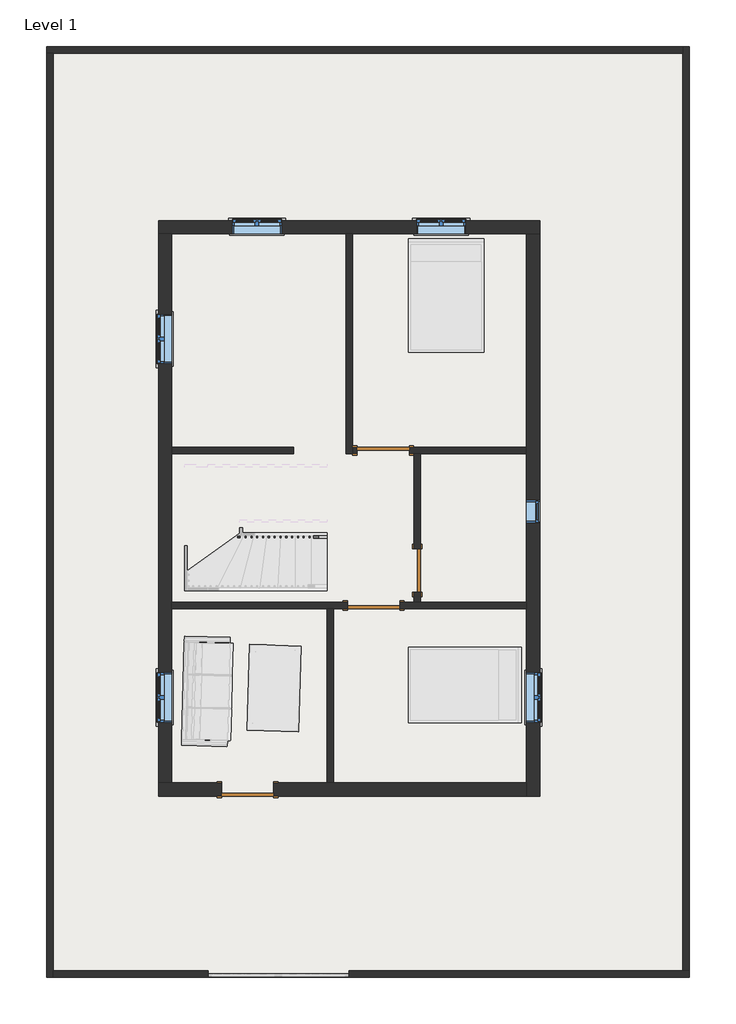
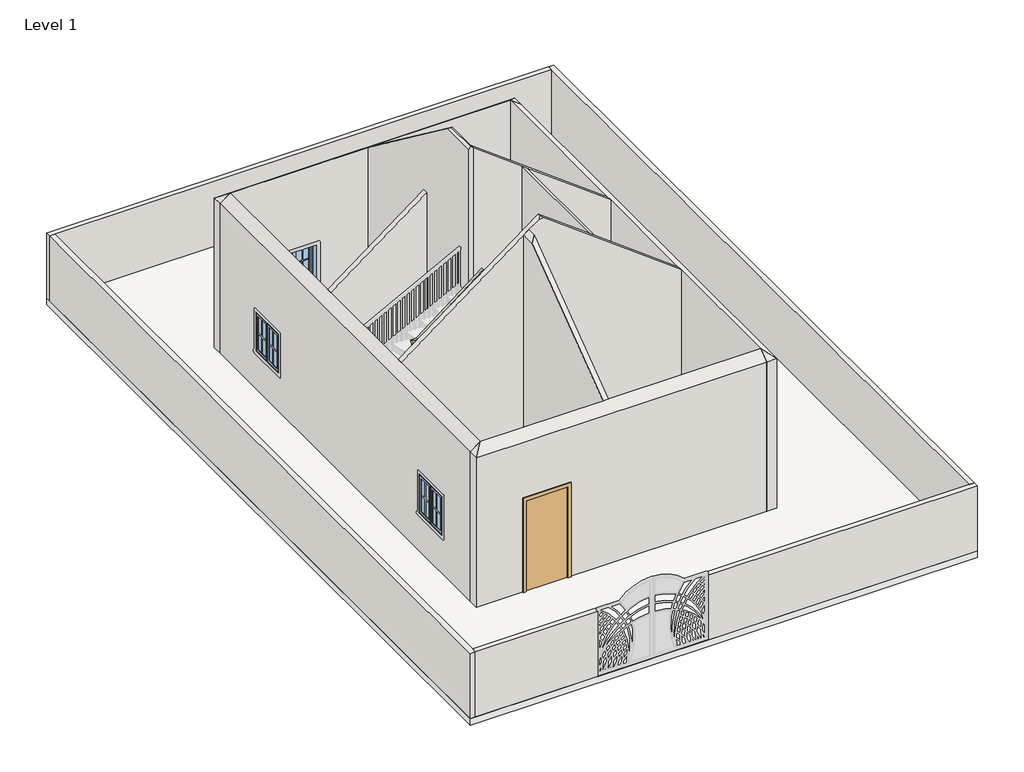
# One storey, part 1 of 2: 15 walls, 6 windows, 4 doors, 1 railing, 1 slab.
"""IFC4 building model written with IfcOpenShell, lengths in millimetres."""

from ifc_helpers import new_model, si_unit, frame, origin, origin_with_axes, place, context, project, spatial, polyline, outline, extrude, faceted_brep, transform, mapped, element, save
from components import door_d8f5dbb5, door_305aa2a5, door_e5f9f3c4, door_0ca8825f, window_aa618e30, window_339605e1

model = new_model("IFC4")

# Units and contexts
model_context = context("Model", 3, world=origin())
ifc_project = project(units=[si_unit("LENGTHUNIT", "METRE", prefix="MILLI")], contexts=[model_context])

# Site, building, storey
site = spatial("IfcSite", under=ifc_project)
building = spatial("IfcBuilding", under=site)
storey = spatial("IfcBuildingStorey", under=building, Name="Level 1", Elevation=0.0)

# Doors
placement = place(None, origin())
door_shape = door_d8f5dbb5(model_context)
element("IfcDoor", 1, ObjectType="Single-Flush : 30\" x 80\"", at=placement, inside=storey, context=model_context, shape_type="MappedRepresentation", body=[
    mapped(door_shape, transform((-82.2715692, -955.3070853, 0.0), x_axis=(0.0, -1.0, 0.0), y_axis=(1.0, 0.0, 0.0), z_axis=(0.0, 0.0, 1.0))),
])
door_2_shape = door_305aa2a5(model_context)
element("IfcDoor", 2, ObjectType="Single-Flush : 36\" x 84\"", at=placement, inside=storey, context=model_context, shape_type="MappedRepresentation", body=[
    mapped(door_2_shape, transform((-677.5332429, 1140.1929147, 0.0), x_axis=(-1.0, 0.0, 0.0), y_axis=(0.0, -1.0, 0.0), z_axis=(0.0, 0.0, 1.0))),
])
door_3_shape = door_e5f9f3c4(model_context)
element("IfcDoor", 3, ObjectType="Single-Flush : 36\" x 84\"", at=placement, inside=storey, context=model_context, shape_type="MappedRepresentation", body=[
    mapped(door_3_shape, transform((-842.6332429, -1564.9070853, 0.0), x_axis=(-1.0, 0.0, 0.0), y_axis=(0.0, -1.0, 0.0), z_axis=(0.0, 0.0, 1.0))),
])
door_4_shape = door_0ca8825f(model_context)
element("IfcDoor", 4, ObjectType="Single-Flush : 36\" x 84\"", at=placement, inside=storey, context=model_context, shape_type="MappedRepresentation", body=[
    mapped(door_4_shape, transform((-3047.6199167, -4784.3570853, 0.0), x_axis=(-1.0, 0.0, 0.0), y_axis=(0.0, -1.0, 0.0), z_axis=(0.0, 0.0, 1.0))),
])

# Railing
element("IfcRailing", 5, ObjectType="Handrail - Rectangular", at=placement, inside=storey, context=model_context, shape_type="SolidModel", body=[
    faceted_brep([(-1660.1449167, -396.5070853, 1083.7333333), (-1660.1449167, -396.5070853, 1019.4000346), (-1660.1449167, -345.7070853, 1019.4000346), (-1660.1449167, -345.7070853, 1083.7333333), (-3111.6766085, -396.5070853, 2211.6191036), (-3162.4766085, -396.5070853, 2186.7590024), (-3162.4766085, -345.7070853, 2186.7590024), (-3111.6766085, -345.7070853, 2211.6191036), (-3111.6766085, -396.5070853, 2414.6281882), (-3162.4766085, -396.5070853, 2363.8281882), (-3162.4766085, -345.7070853, 2363.8281882), (-3111.6766085, -345.7070853, 2414.6281882), (-3238.6766085, -396.5070853, 2414.6281882), (-3238.6766085, -396.5070853, 2363.8281882), (-3187.8766085, -345.7070853, 2363.8281882), (-3187.8766085, -345.7070853, 2414.6281882), (-3238.6766085, -269.5070853, 2414.6281882), (-3238.6766085, -240.3857515, 2363.8281882), (-3187.8766085, -240.3857515, 2363.8281882), (-3187.8766085, -269.5070853, 2414.6281882), (-3238.6766085, -142.5070853, 2631.5051451), (-3238.6766085, -91.7070853, 2617.7256424), (-3187.8766085, -91.7070853, 2617.7256424), (-3187.8766085, -142.5070853, 2631.5051451), (-3238.6766085, -142.5070853, 2834.5142297), (-3238.6766085, -91.7070853, 2783.7142297), (-3187.8766085, -91.7070853, 2783.7142297), (-3187.8766085, -142.5070853, 2834.5142297), (-3238.6766085, -15.5070853, 2834.5142297), (-3238.6766085, -15.5070853, 2783.7142297), (-3187.8766085, -66.3070853, 2783.7142297), (-3187.8766085, -66.3070853, 2834.5142297), (-3111.6766085, -15.5070853, 2834.5142297), (-3094.2599406, -15.5070853, 2783.7142297), (-3094.2599406, -66.3070853, 2783.7142297), (-3111.6766085, -66.3070853, 2834.5142297), (-1660.1449167, -15.5070853, 3962.4), (-1660.1449167, -66.3070853, 3962.4), (-1660.1449167, -66.3070853, 3898.0667013), (-1660.1449167, -15.5070853, 3898.0667013)], [[[0, 1, 2, 3]], [[1, 0, 4, 5]], [[2, 1, 5, 6]], [[3, 2, 6, 7]], [[0, 3, 7, 4]], [[5, 4, 8, 9]], [[6, 5, 9, 10]], [[7, 6, 10, 11]], [[4, 7, 11, 8]], [[9, 8, 12, 13]], [[10, 9, 13, 14]], [[11, 10, 14, 15]], [[8, 11, 15, 12]], [[13, 12, 16, 17]], [[14, 13, 17, 18]], [[15, 14, 18, 19]], [[12, 15, 19, 16]], [[17, 16, 20, 21]], [[18, 17, 21, 22]], [[19, 18, 22, 23]], [[16, 19, 23, 20]], [[21, 20, 24, 25]], [[22, 21, 25, 26]], [[23, 22, 26, 27]], [[20, 23, 27, 24]], [[25, 24, 28, 29]], [[26, 25, 29, 30]], [[27, 26, 30, 31]], [[24, 27, 31, 28]], [[29, 28, 32, 33]], [[30, 29, 33, 34]], [[31, 30, 34, 35]], [[28, 31, 35, 32]], [[36, 37, 38, 39]], [[33, 32, 36, 39]], [[34, 33, 39, 38]], [[35, 34, 38, 37]], [[32, 35, 37, 36]]]),
    extrude(outline(polyline([(3882.8316852, -1679.7516085), (3868.0292361, -1698.8016085), (2878.6666667, -1698.8016085), (2878.6666667, -1679.7516085), (3882.8316852, -1679.7516085)])), frame((0.0, -50.4320853, 0.0), z_axis=(0.0, 1.0, 0.0), x_axis=(0.0, 0.0, 1.0)), (0.0, 0.0, 1.0), 19.05),
    extrude(outline(polyline([(3803.8852902, -1781.3516085), (3789.0828411, -1800.4016085), (2878.6666667, -1800.4016085), (2878.6666667, -1781.3516085), (3803.8852902, -1781.3516085)])), frame((0.0, -50.4320853, 0.0), z_axis=(0.0, 1.0, 0.0), x_axis=(0.0, 0.0, 1.0)), (0.0, 0.0, 1.0), 19.05),
    extrude(outline(polyline([(3724.9388952, -1882.9516085), (3710.1364462, -1902.0016085), (2878.6666667, -1902.0016085), (2878.6666667, -1882.9516085), (3724.9388952, -1882.9516085)])), frame((0.0, -50.4320853, 0.0), z_axis=(0.0, 1.0, 0.0), x_axis=(0.0, 0.0, 1.0)), (0.0, 0.0, 1.0), 19.05),
    extrude(outline(polyline([(3645.9925003, -1984.5516085), (3631.1900512, -2003.6016085), (2709.3333333, -2003.6016085), (2709.3333333, -1984.5516085), (3645.9925003, -1984.5516085)])), frame((0.0, -50.4320853, 0.0), z_axis=(0.0, 1.0, 0.0), x_axis=(0.0, 0.0, 1.0)), (0.0, 0.0, 1.0), 19.05),
    extrude(outline(polyline([(3567.0461053, -2086.1516085), (3552.2436562, -2105.2016085), (2709.3333333, -2105.2016085), (2709.3333333, -2086.1516085), (3567.0461053, -2086.1516085)])), frame((0.0, -50.4320853, 0.0), z_axis=(0.0, 1.0, 0.0), x_axis=(0.0, 0.0, 1.0)), (0.0, 0.0, 1.0), 19.05),
    extrude(outline(polyline([(3488.0997103, -2187.7516085), (3473.2972613, -2206.8016085), (2709.3333333, -2206.8016085), (2709.3333333, -2187.7516085), (3488.0997103, -2187.7516085)])), frame((0.0, -50.4320853, 0.0), z_axis=(0.0, 1.0, 0.0), x_axis=(0.0, 0.0, 1.0)), (0.0, 0.0, 1.0), 19.05),
    extrude(outline(polyline([(3409.1533154, -2289.3516085), (3394.3508663, -2308.4016085), (2540.0, -2308.4016085), (2540.0, -2289.3516085), (3409.1533154, -2289.3516085)])), frame((0.0, -50.4320853, 0.0), z_axis=(0.0, 1.0, 0.0), x_axis=(0.0, 0.0, 1.0)), (0.0, 0.0, 1.0), 19.05),
    extrude(outline(polyline([(3330.2069204, -2390.9516085), (3315.4044713, -2410.0016085), (2540.0, -2410.0016085), (2540.0, -2390.9516085), (3330.2069204, -2390.9516085)])), frame((0.0, -50.4320853, 0.0), z_axis=(0.0, 1.0, 0.0), x_axis=(0.0, 0.0, 1.0)), (0.0, 0.0, 1.0), 19.05),
    extrude(outline(polyline([(3251.2605254, -2492.5516085), (3236.4580764, -2511.6016085), (2370.6666667, -2511.6016085), (2370.6666667, -2492.5516085), (3251.2605254, -2492.5516085)])), frame((0.0, -50.4320853, 0.0), z_axis=(0.0, 1.0, 0.0), x_axis=(0.0, 0.0, 1.0)), (0.0, 0.0, 1.0), 19.05),
    extrude(outline(polyline([(3172.3141304, -2594.1516085), (3157.5116814, -2613.2016085), (2370.6666667, -2613.2016085), (2370.6666667, -2594.1516085), (3172.3141304, -2594.1516085)])), frame((0.0, -50.4320853, 0.0), z_axis=(0.0, 1.0, 0.0), x_axis=(0.0, 0.0, 1.0)), (0.0, 0.0, 1.0), 19.05),
    extrude(outline(polyline([(3093.3677355, -2695.7516085), (3078.5652864, -2714.8016085), (2370.6666667, -2714.8016085), (2370.6666667, -2695.7516085), (3093.3677355, -2695.7516085)])), frame((0.0, -50.4320853, 0.0), z_axis=(0.0, 1.0, 0.0), x_axis=(0.0, 0.0, 1.0)), (0.0, 0.0, 1.0), 19.05),
    extrude(outline(polyline([(3014.4213405, -2797.3516085), (2999.6188914, -2816.4016085), (2201.3333333, -2816.4016085), (2201.3333333, -2797.3516085), (3014.4213405, -2797.3516085)])), frame((0.0, -50.4320853, 0.0), z_axis=(0.0, 1.0, 0.0), x_axis=(0.0, 0.0, 1.0)), (0.0, 0.0, 1.0), 19.05),
    extrude(outline(polyline([(2935.4749455, -2898.9516085), (2920.6724965, -2918.0016085), (2201.3333333, -2918.0016085), (2201.3333333, -2898.9516085), (2935.4749455, -2898.9516085)])), frame((0.0, -50.4320853, 0.0), z_axis=(0.0, 1.0, 0.0), x_axis=(0.0, 0.0, 1.0)), (0.0, 0.0, 1.0), 19.05),
    extrude(outline(polyline([(2856.5285506, -3000.5516085), (2841.7261015, -3019.6016085), (2032.0, -3019.6016085), (2032.0, -3000.5516085), (2856.5285506, -3000.5516085)])), frame((0.0, -50.4320853, 0.0), z_axis=(0.0, 1.0, 0.0), x_axis=(0.0, 0.0, 1.0)), (0.0, 0.0, 1.0), 19.05),
    extrude(outline(polyline([(2777.5821556, -3102.1516085), (2762.7797065, -3121.2016085), (2032.0, -3121.2016085), (2032.0, -3102.1516085), (2777.5821556, -3102.1516085)])), frame((0.0, -50.4320853, 0.0), z_axis=(0.0, 1.0, 0.0), x_axis=(0.0, 0.0, 1.0)), (0.0, 0.0, 1.0), 19.05),
    extrude(outline(polyline([(-3203.7516085, -75.8320853), (-3222.8016085, -75.8320853), (-3222.8016085, -56.7820853), (-3203.7516085, -56.7820853), (-3203.7516085, -75.8320853)])), frame((0.0, 0.0, 1693.3333333), z_axis=(0.0, 0.0, 1.0), x_axis=(1.0, 0.0, 0.0)), (0.0, 0.0, 1.0), 1090.3808964),
    extrude(outline(polyline([(-177.4320853, 2471.3336964), (-158.3820853, 2503.86524), (-158.3820853, 1524.0), (-177.4320853, 1524.0), (-177.4320853, 2471.3336964)])), frame((-3222.8016085, 0.0, 0.0), z_axis=(1.0, 0.0, 0.0), x_axis=(0.0, 1.0, 0.0)), (0.0, 0.0, 1.0), 19.05),
    extrude(outline(polyline([(-279.0320853, 2297.8321309), (-259.9820853, 2330.3636744), (-259.9820853, 1354.6666667), (-279.0320853, 1354.6666667), (-279.0320853, 2297.8321309)])), frame((-3222.8016085, 0.0, 0.0), z_axis=(1.0, 0.0, 0.0), x_axis=(0.0, 1.0, 0.0)), (0.0, 0.0, 1.0), 19.05),
    extrude(outline(polyline([(-3174.6199167, -361.5820853), (-3174.6199167, -380.6320853), (-3193.6699167, -380.6320853), (-3193.6699167, -361.5820853), (-3174.6199167, -361.5820853)])), frame((0.0, 0.0, 1185.3333333), z_axis=(0.0, 0.0, 1.0), x_axis=(1.0, 0.0, 0.0)), (0.0, 0.0, 1.0), 1178.4948549),
    extrude(outline(polyline([(2117.2483397, -3073.0199167), (2132.0507888, -3092.0699167), (1016.0, -3092.0699167), (1016.0, -3073.0199167), (2117.2483397, -3073.0199167)])), frame((0.0, -380.6320853, 0.0), z_axis=(0.0, 1.0, 0.0), x_axis=(0.0, 0.0, 1.0)), (0.0, 0.0, 1.0), 19.05),
    extrude(outline(polyline([(2038.3019447, -2971.4199167), (2053.1043938, -2990.4699167), (1016.0, -2990.4699167), (1016.0, -2971.4199167), (2038.3019447, -2971.4199167)])), frame((0.0, -380.6320853, 0.0), z_axis=(0.0, 1.0, 0.0), x_axis=(0.0, 0.0, 1.0)), (0.0, 0.0, 1.0), 19.05),
    extrude(outline(polyline([(1959.3555498, -2869.8199167), (1974.1579988, -2888.8699167), (846.6666667, -2888.8699167), (846.6666667, -2869.8199167), (1959.3555498, -2869.8199167)])), frame((0.0, -380.6320853, 0.0), z_axis=(0.0, 1.0, 0.0), x_axis=(0.0, 0.0, 1.0)), (0.0, 0.0, 1.0), 19.05),
    extrude(outline(polyline([(1880.4091548, -2768.2199167), (1895.2116039, -2787.2699167), (846.6666667, -2787.2699167), (846.6666667, -2768.2199167), (1880.4091548, -2768.2199167)])), frame((0.0, -380.6320853, 0.0), z_axis=(0.0, 1.0, 0.0), x_axis=(0.0, 0.0, 1.0)), (0.0, 0.0, 1.0), 19.05),
    extrude(outline(polyline([(1801.4627598, -2666.6199167), (1816.2652089, -2685.6699167), (677.3333333, -2685.6699167), (677.3333333, -2666.6199167), (1801.4627598, -2666.6199167)])), frame((0.0, -380.6320853, 0.0), z_axis=(0.0, 1.0, 0.0), x_axis=(0.0, 0.0, 1.0)), (0.0, 0.0, 1.0), 19.05),
    extrude(outline(polyline([(1722.5163649, -2565.0199167), (1737.3188139, -2584.0699167), (677.3333333, -2584.0699167), (677.3333333, -2565.0199167), (1722.5163649, -2565.0199167)])), frame((0.0, -380.6320853, 0.0), z_axis=(0.0, 1.0, 0.0), x_axis=(0.0, 0.0, 1.0)), (0.0, 0.0, 1.0), 19.05),
    extrude(outline(polyline([(1643.5699699, -2463.4199167), (1658.3724189, -2482.4699167), (508.0, -2482.4699167), (508.0, -2463.4199167), (1643.5699699, -2463.4199167)])), frame((0.0, -380.6320853, 0.0), z_axis=(0.0, 1.0, 0.0), x_axis=(0.0, 0.0, 1.0)), (0.0, 0.0, 1.0), 19.05),
    extrude(outline(polyline([(1564.6235749, -2361.8199167), (1579.426024, -2380.8699167), (508.0, -2380.8699167), (508.0, -2361.8199167), (1564.6235749, -2361.8199167)])), frame((0.0, -380.6320853, 0.0), z_axis=(0.0, 1.0, 0.0), x_axis=(0.0, 0.0, 1.0)), (0.0, 0.0, 1.0), 19.05),
    extrude(outline(polyline([(1485.6771799, -2260.2199167), (1500.479629, -2279.2699167), (508.0, -2279.2699167), (508.0, -2260.2199167), (1485.6771799, -2260.2199167)])), frame((0.0, -380.6320853, 0.0), z_axis=(0.0, 1.0, 0.0), x_axis=(0.0, 0.0, 1.0)), (0.0, 0.0, 1.0), 19.05),
    extrude(outline(polyline([(1406.730785, -2158.6199167), (1421.533234, -2177.6699167), (338.6666667, -2177.6699167), (338.6666667, -2158.6199167), (1406.730785, -2158.6199167)])), frame((0.0, -380.6320853, 0.0), z_axis=(0.0, 1.0, 0.0), x_axis=(0.0, 0.0, 1.0)), (0.0, 0.0, 1.0), 19.05),
    extrude(outline(polyline([(1327.78439, -2057.0199167), (1342.5868391, -2076.0699167), (338.6666667, -2076.0699167), (338.6666667, -2057.0199167), (1327.78439, -2057.0199167)])), frame((0.0, -380.6320853, 0.0), z_axis=(0.0, 1.0, 0.0), x_axis=(0.0, 0.0, 1.0)), (0.0, 0.0, 1.0), 19.05),
    extrude(outline(polyline([(1248.837995, -1955.4199167), (1263.6404441, -1974.4699167), (338.6666667, -1974.4699167), (338.6666667, -1955.4199167), (1248.837995, -1955.4199167)])), frame((0.0, -380.6320853, 0.0), z_axis=(0.0, 1.0, 0.0), x_axis=(0.0, 0.0, 1.0)), (0.0, 0.0, 1.0), 19.05),
    extrude(outline(polyline([(1169.8916001, -1853.8199167), (1184.6940491, -1872.8699167), (169.3333333, -1872.8699167), (169.3333333, -1853.8199167), (1169.8916001, -1853.8199167)])), frame((0.0, -380.6320853, 0.0), z_axis=(0.0, 1.0, 0.0), x_axis=(0.0, 0.0, 1.0)), (0.0, 0.0, 1.0), 19.05),
    extrude(outline(polyline([(1090.9452051, -1752.2199167), (1105.7476541, -1771.2699167), (169.3333333, -1771.2699167), (169.3333333, -1752.2199167), (1090.9452051, -1752.2199167)])), frame((0.0, -380.6320853, 0.0), z_axis=(0.0, 1.0, 0.0), x_axis=(0.0, 0.0, 1.0)), (0.0, 0.0, 1.0), 19.05),
    extrude(outline(polyline([(-3203.7516085, -50.4320853), (-3222.8016085, -50.4320853), (-3222.8016085, -31.3820853), (-3203.7516085, -31.3820853), (-3203.7516085, -50.4320853)])), frame((0.0, 0.0, 1862.6666667), z_axis=(0.0, 0.0, 1.0), x_axis=(1.0, 0.0, 0.0)), (0.0, 0.0, 1.0), 921.0475631),
    extrude(outline(polyline([(-3203.7516085, -361.5820853), (-3203.7516085, -380.6320853), (-3222.8016085, -380.6320853), (-3222.8016085, -361.5820853), (-3203.7516085, -361.5820853)])), frame((0.0, 0.0, 1185.3333333), z_axis=(0.0, 0.0, 1.0), x_axis=(1.0, 0.0, 0.0)), (0.0, 0.0, 1.0), 1178.4948549),
    extrude(outline(polyline([(3898.0667013, -1660.1449167), (3883.2642523, -1679.1949167), (2878.6666667, -1679.1949167), (2878.6666667, -1660.1449167), (3898.0667013, -1660.1449167)])), frame((0.0, -50.4320853, 0.0), z_axis=(0.0, 1.0, 0.0), x_axis=(0.0, 0.0, 1.0)), (0.0, 0.0, 1.0), 19.05),
    extrude(outline(polyline([(1019.4000346, -1660.1449167), (1034.2024837, -1679.1949167), (169.3333333, -1679.1949167), (169.3333333, -1660.1449167), (1019.4000346, -1660.1449167)])), frame((0.0, -380.6320853, 0.0), z_axis=(0.0, 1.0, 0.0), x_axis=(0.0, 0.0, 1.0)), (0.0, 0.0, 1.0), 19.05),
])

# Slab
element("IfcSlab", 6, ObjectType="Generic - 12\"", at=placement, inside=storey, context=model_context, shape_type="SweptSolid", body=[
    extrude(outline(polyline([(4675.3638952, 8200.4974943), (4675.3638952, -8068.2025057), (-6564.1361048, -8068.2025057), (-6564.1361048, 8200.4974943), (4675.3638952, 8200.4974943)])), frame((0.0, 0.0, -152.4), z_axis=(0.0, 0.0, 1.0), x_axis=(1.0, 0.0, 0.0)), (0.0, 0.0, 1.0), 152.4),
])

# Walls
element("IfcWall", 7, ObjectType="WALL4.5\"", at=placement, inside=storey, context=model_context, shape_type="Brep", body=[
    faceted_brep([(-1329.9449167, 4931.1429147, 0.0), (-1329.9449167, 1083.0429147, 0.0), (-1329.9449167, 1083.0429147, 5962.65), (-1329.9449167, 1883.1429147, 5962.65), (-1329.9449167, 4931.1429147, 3676.65), (-1215.6449167, 4931.1429147, 0.0), (-1215.6449167, 4931.1429147, 3676.65), (-1215.6449167, 1883.1429147, 5962.65), (-1215.6449167, 1197.3429147, 5962.65), (-1215.6449167, 1083.0429147, 5962.65), (-1215.6449167, 1083.0429147, 0.0), (-1215.6449167, 1197.3429147, 0.0), (-1272.7949167, 1083.0429147, 6005.5125), (-1272.7949167, 1825.9929147, 6005.5125)], [[[0, 1, 2, 3, 4]], [[5, 6, 7, 8, 9, 10, 11]], [[1, 0, 5, 11, 10]], [[0, 4, 6, 5]], [[2, 1, 10, 9, 12]], [[4, 3, 13, 7, 6]], [[3, 2, 12, 13]], [[12, 9, 8, 7, 13]]]),
])
element("IfcWall", 8, ObjectType="WALL4.5\"", at=placement, inside=storey, context=model_context, shape_type="Brep", body=[
    faceted_brep([(-1215.6449167, 1083.0429147, 0.0), (-1134.7332429, 1083.0429147, 0.0), (-1134.7332429, 1083.0429147, 2133.6), (-220.3332429, 1083.0429147, 2133.6), (-220.3332429, 1083.0429147, 0.0), (-139.4215692, 1083.0429147, 0.0), (-25.1215692, 1083.0429147, 0.0), (1832.3550833, 1083.0429147, 0.0), (1832.3550833, 1083.0429147, 3676.65), (-25.1215692, 1083.0429147, 5069.7574894), (-139.4215692, 1083.0429147, 5155.4824894), (-1215.6449167, 1083.0429147, 5962.65), (-1134.7332429, 1197.3429147, 2133.6), (-1134.7332429, 1197.3429147, 0.0), (-1215.6449167, 1197.3429147, 0.0), (-1215.6449167, 1197.3429147, 5962.65), (1832.3550833, 1197.3429147, 3676.65), (1832.3550833, 1197.3429147, 0.0), (-220.3332429, 1197.3429147, 0.0), (-220.3332429, 1197.3429147, 2133.6)], [[[0, 1, 2, 3, 4, 5, 6, 7, 8, 9, 10, 11]], [[12, 13, 14, 15, 16, 17, 18, 19]], [[18, 17, 7, 6, 5, 4]], [[14, 13, 1, 0]], [[0, 11, 15, 14]], [[8, 7, 17, 16]], [[2, 1, 13, 12]], [[3, 2, 12, 19]], [[4, 3, 19, 18]], [[11, 10, 9, 8, 16, 15]]]),
])
element("IfcWall", 9, ObjectType="WALL4.5\"", at=placement, inside=storey, context=model_context, shape_type="SweptSolid", body=[
    extrude(outline(polyline([(0.0, -4377.9449167), (0.0, -2244.3449167), (5276.85, -2244.3449167), (3676.65, -4377.9449167), (0.0, -4377.9449167)])), frame((0.0, 1083.0429147, 0.0), z_axis=(0.0, 1.0, 0.0), x_axis=(0.0, 0.0, 1.0)), (0.0, 0.0, 1.0), 114.3),
])
element("IfcWall", 10, ObjectType="WALL4.5\"", at=placement, inside=storey, context=model_context, shape_type="Brep", body=[
    faceted_brep([(-139.4215692, -1336.3070853, 2032.0), (-139.4215692, -1336.3070853, 0.0), (-139.4215692, -1507.7570853, 0.0), (-139.4215692, -1507.7570853, 5155.4824894), (-139.4215692, 1083.0429147, 5155.4824894), (-139.4215692, 1083.0429147, 0.0), (-139.4215692, -574.3070853, 0.0), (-139.4215692, -574.3070853, 2032.0), (-25.1215692, -1507.7570853, 0.0), (-25.1215692, -1336.3070853, 0.0), (-25.1215692, -1336.3070853, 2032.0), (-25.1215692, -574.3070853, 2032.0), (-25.1215692, -574.3070853, 0.0), (-25.1215692, 1083.0429147, 0.0), (-25.1215692, 1083.0429147, 5069.7574894), (-25.1215692, -1507.7570853, 5069.7574894)], [[[0, 1, 2, 3, 4, 5, 6, 7]], [[8, 9, 10, 11, 12, 13, 14, 15]], [[6, 5, 13, 12]], [[2, 1, 9, 8]], [[5, 4, 14, 13]], [[3, 2, 8, 15]], [[10, 9, 1, 0]], [[11, 10, 0, 7]], [[12, 11, 7, 6]], [[4, 3, 15, 14]]]),
])
element("IfcWall", 11, ObjectType="WALL4.5\"", at=placement, inside=storey, context=model_context, shape_type="Brep", body=[
    faceted_brep([(-4377.9449167, -1622.0570853, 0.0), (-1660.1449167, -1622.0570853, 0.0), (-1545.8449167, -1622.0570853, 0.0), (-1299.8332429, -1622.0570853, 0.0), (-1299.8332429, -1622.0570853, 2133.6), (-385.4332429, -1622.0570853, 2133.6), (-385.4332429, -1622.0570853, 0.0), (1832.3550833, -1622.0570853, 0.0), (1832.3550833, -1622.0570853, 3676.65), (-1215.6449167, -1622.0570853, 5962.65), (-1329.9449167, -1622.0570853, 5962.65), (-1545.8449167, -1622.0570853, 5800.725), (-1660.1449167, -1622.0570853, 5715.0), (-4377.9449167, -1622.0570853, 3676.65), (-1299.8332429, -1507.7570853, 2133.6), (-1299.8332429, -1507.7570853, 0.0), (-4377.9449167, -1507.7570853, 0.0), (-4377.9449167, -1507.7570853, 3676.65), (-1272.7949167, -1507.7570853, 6005.5125), (-139.4215692, -1507.7570853, 5155.4824894), (-25.1215692, -1507.7570853, 5069.7574894), (1832.3550833, -1507.7570853, 3676.65), (1832.3550833, -1507.7570853, 0.0), (-25.1215692, -1507.7570853, 0.0), (-139.4215692, -1507.7570853, 0.0), (-385.4332429, -1507.7570853, 0.0), (-385.4332429, -1507.7570853, 2133.6), (-1272.7949167, -1564.9070853, 6005.5125)], [[[0, 1, 2, 3, 4, 5, 6, 7, 8, 9, 10, 11, 12, 13]], [[14, 15, 16, 17, 18, 19, 20, 21, 22, 23, 24, 25, 26]], [[16, 15, 3, 2, 1, 0]], [[25, 24, 23, 22, 7, 6]], [[8, 7, 22, 21]], [[0, 13, 17, 16]], [[4, 3, 15, 14]], [[5, 4, 14, 26]], [[6, 5, 26, 25]], [[13, 12, 11, 10, 27, 18, 17]], [[10, 9, 27]], [[9, 8, 21, 20, 19, 18, 27]]]),
])
element("IfcWall", 12, ObjectType="WALL4.5\"", at=placement, inside=storey, context=model_context, shape_type="Brep", body=[
    faceted_brep([(-1660.1449167, -1622.0570853, 0.0), (-1660.1449167, -4670.0570853, 0.0), (-1660.1449167, -4670.0570853, 3676.65), (-1660.1449167, -1952.2570853, 5715.0), (-1660.1449167, -1622.0570853, 5715.0), (-1545.8449167, -1622.0570853, 0.0), (-1545.8449167, -1622.0570853, 5800.725), (-1545.8449167, -1837.9570853, 5800.725), (-1545.8449167, -4670.0570853, 3676.65), (-1545.8449167, -4670.0570853, 0.0)], [[[0, 1, 2, 3, 4]], [[5, 6, 7, 8, 9]], [[1, 0, 5, 9]], [[2, 1, 9, 8]], [[0, 4, 6, 5]], [[4, 3, 7, 6]], [[3, 2, 8, 7]]]),
])
element("IfcWall", 13, ObjectType="WALL4.5\"", at=placement, inside=storey, context=model_context, shape_type="Brep", body=[
    faceted_brep([(-6564.1361048, 8086.1974943, 0.0), (-6449.8361048, 8086.1974943, 0.0), (4561.0638952, 8086.1974943, 0.0), (4561.0638952, 8086.1974943, 1524.0), (-6449.8361048, 8086.1974943, 1524.0), (-6564.1361048, 8086.1974943, 1524.0), (-6564.1361048, 8200.4974943, 0.0), (-6564.1361048, 8200.4974943, 1524.0), (4561.0638952, 8200.4974943, 1524.0), (4561.0638952, 8200.4974943, 0.0)], [[[0, 1, 2, 3, 4, 5]], [[6, 7, 8, 9]], [[2, 1, 0, 6, 9]], [[5, 4, 3, 8, 7]], [[0, 5, 7, 6]], [[3, 2, 9, 8]]]),
])
element("IfcWall", 14, ObjectType="WALL4.5\"", at=placement, inside=storey, context=model_context, shape_type="Brep", body=[
    faceted_brep([(-6449.8361048, -8068.2025057, 0.0), (-6449.8361048, -7953.9025057, 0.0), (-6449.8361048, 8086.1974943, 0.0), (-6449.8361048, 8086.1974943, 1524.0), (-6449.8361048, -7953.9025057, 1524.0), (-6449.8361048, -8068.2025057, 1524.0), (-6564.1361048, -8068.2025057, 0.0), (-6564.1361048, -8068.2025057, 1524.0), (-6564.1361048, 8086.1974943, 1524.0), (-6564.1361048, 8086.1974943, 0.0)], [[[0, 1, 2, 3, 4, 5]], [[6, 7, 8, 9]], [[2, 1, 0, 6, 9]], [[5, 4, 3, 8, 7]], [[0, 5, 7, 6]], [[3, 2, 9, 8]]]),
])
element("IfcWall", 15, ObjectType="WALL4.5\"", at=placement, inside=storey, context=model_context, shape_type="Brep", body=[
    faceted_brep([(4675.3638952, -7953.9025057, 0.0), (4561.0638952, -7953.9025057, 0.0), (-1274.5861048, -7953.9025057, 0.0), (-1274.5861048, -7953.9025057, 1524.0), (4561.0638952, -7953.9025057, 1524.0), (4675.3638952, -7953.9025057, 1524.0), (4675.3638952, -8068.2025057, 0.0), (4675.3638952, -8068.2025057, 1524.0), (-1274.5861048, -8068.2025057, 1524.0), (-1274.5861048, -8068.2025057, 0.0)], [[[0, 1, 2, 3, 4, 5]], [[6, 7, 8, 9]], [[2, 1, 0, 6, 9]], [[3, 2, 9, 8]], [[5, 4, 3, 8, 7]], [[0, 5, 7, 6]]]),
])
element("IfcWall", 16, ObjectType="WALL4.5\"", at=placement, inside=storey, context=model_context, shape_type="Brep", body=[
    faceted_brep([(4561.0638952, 8200.4974943, 0.0), (4561.0638952, 8086.1974943, 0.0), (4561.0638952, -7953.9025057, 0.0), (4561.0638952, -7953.9025057, 1524.0), (4561.0638952, 8086.1974943, 1524.0), (4561.0638952, 8200.4974943, 1524.0), (4675.3638952, 8200.4974943, 0.0), (4675.3638952, 8200.4974943, 1524.0), (4675.3638952, -7953.9025057, 1524.0), (4675.3638952, -7953.9025057, 0.0)], [[[0, 1, 2, 3, 4, 5]], [[6, 7, 8, 9]], [[2, 1, 0, 6, 9]], [[5, 4, 3, 8, 7]], [[0, 5, 7, 6]], [[3, 2, 9, 8]]]),
])
element("IfcWall", 17, ObjectType="WALL4.5\"", at=placement, inside=storey, context=model_context, shape_type="SweptSolid", body=[
    extrude(outline(polyline([(-6449.8361048, -7953.9025057), (-3739.7699167, -7953.9025057), (-3739.7699167, -8068.2025057), (-6449.8361048, -8068.2025057), (-6449.8361048, -7953.9025057)])), origin_with_axes(), (0.0, 0.0, 1.0), 1524.0),
])
element("IfcWall", 18, ObjectType="WALL9\"", at=placement, inside=storey, context=model_context, shape_type="Brep", body=[
    faceted_brep([(-4606.5449167, 4931.1429147, 0.0), (-4377.9449167, 4931.1429147, 0.0), (-1329.9449167, 4931.1429147, 0.0), (-1215.6449167, 4931.1429147, 0.0), (1832.3550833, 4931.1429147, 0.0), (2060.9550833, 4931.1429147, 0.0), (2060.9550833, 4931.1429147, 3505.2), (1832.3550833, 4931.1429147, 3676.65), (-1215.6449167, 4931.1429147, 3676.65), (-1329.9449167, 4931.1429147, 3676.65), (-4377.9449167, 4931.1429147, 3676.65), (-4606.5449167, 4931.1429147, 3505.2), (-2450.7199167, 4931.1429147, 1828.8), (-2450.7199167, 4931.1429147, 914.4), (-3314.3199167, 4931.1429147, 914.4), (-3314.3199167, 4931.1429147, 1828.8), (768.7300833, 4931.1429147, 1828.8), (768.7300833, 4931.1429147, 914.4), (-94.8699167, 4931.1429147, 914.4), (-94.8699167, 4931.1429147, 1828.8), (-4606.5449167, 5159.7429147, 0.0), (-4606.5449167, 5159.7429147, 3505.2), (2060.9550833, 5159.7429147, 3505.2), (2060.9550833, 5159.7429147, 0.0), (-2450.7199167, 5159.7429147, 1828.8), (-3314.3199167, 5159.7429147, 1828.8), (-3314.3199167, 5159.7429147, 914.4), (-2450.7199167, 5159.7429147, 914.4), (768.7300833, 5159.7429147, 1828.8), (-94.8699167, 5159.7429147, 1828.8), (-94.8699167, 5159.7429147, 914.4), (768.7300833, 5159.7429147, 914.4)], [[[0, 1, 2, 3, 4, 5, 6, 7, 8, 9, 10, 11], [12, 13, 14, 15], [16, 17, 18, 19]], [[20, 21, 22, 23], [24, 25, 26, 27], [28, 29, 30, 31]], [[5, 4, 3, 2, 1, 0, 20, 23]], [[6, 5, 23, 22]], [[0, 11, 21, 20]], [[13, 12, 24, 27]], [[14, 13, 27, 26]], [[15, 14, 26, 25]], [[12, 15, 25, 24]], [[17, 16, 28, 31]], [[18, 17, 31, 30]], [[19, 18, 30, 29]], [[16, 19, 29, 28]], [[11, 10, 21]], [[10, 9, 8, 7, 22, 21]], [[7, 6, 22]]]),
])
element("IfcWall", 19, ObjectType="WALL9\"", at=placement, inside=storey, context=model_context, shape_type="Brep", body=[
    faceted_brep([(1832.3550833, 4931.1429147, 0.0), (1832.3550833, 1197.3429147, 0.0), (1832.3550833, 1083.0429147, 0.0), (1832.3550833, -1507.7570853, 0.0), (1832.3550833, -1622.0570853, 0.0), (1832.3550833, -4670.0570853, 0.0), (1832.3550833, -4898.6570853, 0.0), (1832.3550833, -4898.6570853, 3505.2), (1832.3550833, -4670.0570853, 3676.65), (1832.3550833, -1622.0570853, 3676.65), (1832.3550833, -1507.7570853, 3676.65), (1832.3550833, 1083.0429147, 3676.65), (1832.3550833, 1197.3429147, 3676.65), (1832.3550833, 4931.1429147, 3676.65), (1832.3550833, -129.8070853, 1524.0), (1832.3550833, -129.8070853, 914.4), (1832.3550833, 276.5929147, 914.4), (1832.3550833, 276.5929147, 1524.0), (1832.3550833, -3606.4320853, 1828.8), (1832.3550833, -3606.4320853, 914.4), (1832.3550833, -2742.8320853, 914.4), (1832.3550833, -2742.8320853, 1828.8), (2060.9550833, 4931.1429147, 0.0), (2060.9550833, 4931.1429147, 3505.2), (2060.9550833, -4898.6570853, 3505.2), (2060.9550833, -4898.6570853, 0.0), (2060.9550833, -129.8070853, 1524.0), (2060.9550833, 276.5929147, 1524.0), (2060.9550833, 276.5929147, 914.4), (2060.9550833, -129.8070853, 914.4), (2060.9550833, -3606.4320853, 1828.8), (2060.9550833, -2742.8320853, 1828.8), (2060.9550833, -2742.8320853, 914.4), (2060.9550833, -3606.4320853, 914.4)], [[[0, 1, 2, 3, 4, 5, 6, 7, 8, 9, 10, 11, 12, 13], [14, 15, 16, 17], [18, 19, 20, 21]], [[22, 23, 24, 25], [26, 27, 28, 29], [30, 31, 32, 33]], [[6, 5, 4, 3, 2, 1, 0, 22, 25]], [[0, 13, 23, 22]], [[7, 6, 25, 24]], [[15, 14, 26, 29]], [[16, 15, 29, 28]], [[17, 16, 28, 27]], [[14, 17, 27, 26]], [[19, 18, 30, 33]], [[20, 19, 33, 32]], [[21, 20, 32, 31]], [[18, 21, 31, 30]], [[13, 12, 11, 10, 9, 8, 24, 23]], [[8, 7, 24]]]),
])
element("IfcWall", 20, ObjectType="WALL9\"", at=placement, inside=storey, context=model_context, shape_type="Brep", body=[
    faceted_brep([(-3504.8199167, -4670.0570853, 2133.6), (-3504.8199167, -4670.0570853, 0.0), (-4377.9449167, -4670.0570853, 0.0), (-4606.5449167, -4670.0570853, 0.0), (-4606.5449167, -4670.0570853, 3505.2), (-4377.9449167, -4670.0570853, 3676.65), (-1660.1449167, -4670.0570853, 3676.65), (-1545.8449167, -4670.0570853, 3676.65), (1832.3550833, -4670.0570853, 3676.65), (1832.3550833, -4670.0570853, 0.0), (-1545.8449167, -4670.0570853, 0.0), (-1660.1449167, -4670.0570853, 0.0), (-2590.4199167, -4670.0570853, 0.0), (-2590.4199167, -4670.0570853, 2133.6), (-4606.5449167, -4898.6570853, 0.0), (-3504.8199167, -4898.6570853, 0.0), (-3504.8199167, -4898.6570853, 2133.6), (-2590.4199167, -4898.6570853, 2133.6), (-2590.4199167, -4898.6570853, 0.0), (1832.3550833, -4898.6570853, 0.0), (1832.3550833, -4898.6570853, 3505.2), (-4606.5449167, -4898.6570853, 3505.2)], [[[0, 1, 2, 3, 4, 5, 6, 7, 8, 9, 10, 11, 12, 13]], [[14, 15, 16, 17, 18, 19, 20, 21]], [[3, 2, 1, 15, 14]], [[12, 11, 10, 9, 19, 18]], [[9, 8, 20, 19]], [[4, 3, 14, 21]], [[16, 15, 1, 0]], [[17, 16, 0, 13]], [[18, 17, 13, 12]], [[8, 7, 6, 5, 21, 20]], [[5, 4, 21]]]),
])
element("IfcWall", 21, ObjectType="WALL9\"", at=placement, inside=storey, context=model_context, shape_type="Brep", body=[
    faceted_brep([(-4377.9449167, -4670.0570853, 0.0), (-4377.9449167, -1622.0570853, 0.0), (-4377.9449167, -1507.7570853, 0.0), (-4377.9449167, 1083.0429147, 0.0), (-4377.9449167, 1197.3429147, 0.0), (-4377.9449167, 4931.1429147, 0.0), (-4377.9449167, 4931.1429147, 3676.65), (-4377.9449167, 1197.3429147, 3676.65), (-4377.9449167, 1083.0429147, 3676.65), (-4377.9449167, -1507.7570853, 3676.65), (-4377.9449167, -1622.0570853, 3676.65), (-4377.9449167, -4670.0570853, 3676.65), (-4377.9449167, 3524.6179147, 1828.8), (-4377.9449167, 3524.6179147, 914.4), (-4377.9449167, 2661.0179147, 914.4), (-4377.9449167, 2661.0179147, 1828.8), (-4377.9449167, -2742.8320853, 1828.8), (-4377.9449167, -2742.8320853, 914.4), (-4377.9449167, -3606.4320853, 914.4), (-4377.9449167, -3606.4320853, 1828.8), (-4606.5449167, -4670.0570853, 0.0), (-4606.5449167, -4670.0570853, 3505.2), (-4606.5449167, 4931.1429147, 3505.2), (-4606.5449167, 4931.1429147, 0.0), (-4606.5449167, 3524.6179147, 1828.8), (-4606.5449167, 2661.0179147, 1828.8), (-4606.5449167, 2661.0179147, 914.4), (-4606.5449167, 3524.6179147, 914.4), (-4606.5449167, -2742.8320853, 1828.8), (-4606.5449167, -3606.4320853, 1828.8), (-4606.5449167, -3606.4320853, 914.4), (-4606.5449167, -2742.8320853, 914.4)], [[[0, 1, 2, 3, 4, 5, 6, 7, 8, 9, 10, 11], [12, 13, 14, 15], [16, 17, 18, 19]], [[20, 21, 22, 23], [24, 25, 26, 27], [28, 29, 30, 31]], [[5, 4, 3, 2, 1, 0, 20, 23]], [[0, 11, 21, 20]], [[6, 5, 23, 22]], [[13, 12, 24, 27]], [[14, 13, 27, 26]], [[15, 14, 26, 25]], [[12, 15, 25, 24]], [[17, 16, 28, 31]], [[18, 17, 31, 30]], [[19, 18, 30, 29]], [[16, 19, 29, 28]], [[11, 10, 9, 8, 7, 6, 22, 21]]]),
])

# Windows
window_shape = window_aa618e30(model_context)
element("IfcWindow", 22, ObjectType="Fixed : 16\" x 24\"", at=placement, inside=storey, context=model_context, shape_type="MappedRepresentation", body=[
    mapped(window_shape, transform((1946.6550833, 35.2929147, 0.0), x_axis=(0.0, -1.0, 0.0), y_axis=(1.0, 0.0, 0.0), z_axis=(0.0, 0.0, 1.0))),
])
window_2_shape = window_339605e1(model_context)
element("IfcWindow", 23, ObjectType="Window-Casement-Double : 34\" x 36\"", at=placement, inside=storey, context=model_context, shape_type="MappedRepresentation", body=[
    mapped(window_2_shape, transform((-2882.5199167, 5045.4429147, 0.0), x_axis=(1.0, 0.0, 0.0), y_axis=(0.0, 1.0, 0.0), z_axis=(0.0, 0.0, 1.0))),
])
element("IfcWindow", 24, ObjectType="Window-Casement-Double : 34\" x 36\"", at=placement, inside=storey, context=model_context, shape_type="MappedRepresentation", body=[
    mapped(window_2_shape, transform((336.9300833, 5045.4429147, 0.0), x_axis=(1.0, 0.0, 0.0), y_axis=(0.0, 1.0, 0.0), z_axis=(0.0, 0.0, 1.0))),
])
element("IfcWindow", 25, ObjectType="Window-Casement-Double : 34\" x 36\"", at=placement, inside=storey, context=model_context, shape_type="MappedRepresentation", body=[
    mapped(window_2_shape, transform((1946.6550833, -3174.6320853, 0.0), x_axis=(0.0, -1.0, 0.0), y_axis=(1.0, 0.0, 0.0), z_axis=(0.0, 0.0, 1.0))),
])
element("IfcWindow", 26, ObjectType="Window-Casement-Double : 34\" x 36\"", at=placement, inside=storey, context=model_context, shape_type="MappedRepresentation", body=[
    mapped(window_2_shape, transform((-4492.2449167, 3092.8179147, 0.0), x_axis=(0.0, 1.0, 0.0), y_axis=(-1.0, 0.0, 0.0), z_axis=(0.0, 0.0, 1.0))),
])
element("IfcWindow", 27, ObjectType="Window-Casement-Double : 34\" x 36\"", at=placement, inside=storey, context=model_context, shape_type="MappedRepresentation", body=[
    mapped(window_2_shape, transform((-4492.2449167, -3174.6320853, 0.0), x_axis=(0.0, 1.0, 0.0), y_axis=(-1.0, 0.0, 0.0), z_axis=(0.0, 0.0, 1.0))),
])

save(model, "model.ifc")

# Revit data of these elements
# Type "Single-Flush : 30\" x 80\""
#   Type Mark = "5"
#   Construction Type Id = "MDOOR"
#   Assembly Code = "C1020"
#   Analytic Construction = "Metal"
#   Thickness = 0' - 2"
#   Heat Transfer Coefficient (U) = 0.651978 BTU/(h·ft²·°F)
#   Height = 6' - 8"
#   Trim Projection Ext = 0' - 1"
#   Trim Projection Int = 0' - 1"
#   Trim Width = 0' - 3"
#   Width = 2' - 6"
#   Define Thermal Properties by = 1
#   Define Thermal Properties by = 1
#   Door Material = Door - Panel
#   Frame Material = Door - Frame
#   Visual Light Transmittance = 0
#   Solar Heat Gain Coefficient = 0
#   Function = (empty or 0)
#   Wall Closure = (empty or 0)
# Type "Single-Flush : 36\" x 84\""
#   Type Mark = "1"
#   Construction Type Id = "MDOOR"
#   Assembly Code = "C1020"
#   Analytic Construction = "Metal"
#   Thickness = 0' - 2"
#   Heat Transfer Coefficient (U) = 0.651978 BTU/(h·ft²·°F)
#   Height = 7' - 0"
#   Trim Projection Ext = 0' - 1"
#   Trim Projection Int = 0' - 1"
#   Trim Width = 0' - 3"
#   Width = 3' - 0"
#   Define Thermal Properties by = 1
#   Define Thermal Properties by = 1
#   Door Material = Door - Panel
#   Frame Material = Door - Frame
#   Visual Light Transmittance = 0
#   Solar Heat Gain Coefficient = 0
#   Function = (empty or 0)
#   Wall Closure = (empty or 0)
# Type "Handrail - Rectangular"
#   Assembly Code = "C2010400"
#   built-in parameter 1008612 = 0.0416667 (stored number, unit not read)
#   built-in parameter 1008611 = 0.0416667 (stored number, unit not read)
#   built-in parameter 1008609 = 0.333333 (stored number, unit not read)
#   built-in parameter 1008604 = 0.166667 (stored number, unit not read)
#   built-in parameter 1008603 = 0.166667 (stored number, unit not read)
#   Railing Height = 3' - 0"
#   built-in parameter 1008630 = 2
#   built-in parameter 1008610 = 2
#   built-in parameter 1008618 = Baluster - Square : 3/4"
# Type "Generic - 12\""
#   Assembly Code = "B1010"
#   Function = 0
#   Layers, outside or top first: 0' - 6" no material (function 1)
# Type "WALL4.5\""
#   Assembly Code = "B2010"
#   Layers, outside or top first: 0' - 4 1/2" no material (function 1)
# Type "WALL9\""
#   Assembly Code = "B2010"
#   Layers, outside or top first: 0' - 9" no material (function 1)
# Type "Fixed : 16\" x 24\""
#   Type Mark = "4"
#   Construction Type Id = "GSP4R"
#   Assembly Code = "B2020100"
#   Analytic Construction = "1/8 in Pilkington single glazing"
#   Visual Light Transmittance = 0.9
#   Solar Heat Gain Coefficient = 0.78
#   Heat Transfer Coefficient (U) = 0.6496 BTU/(h·ft²·°F)
#   Height = 2' - 0"
#   Default Sill Height = 3' - 0"
#   Width = 1' - 4"
#   Window Inset = 0' - 0 3/4"
#   Define Thermal Properties by = 1
#   Define Thermal Properties by = 1
#   Glass Pane Material = Glass
#   Sash Material = Sash
#   Wall Closure = (empty or 0)
# Type "Window-Casement-Double : 34\" x 36\""
#   Type Mark = "14"
#   Fire Rating = "0.5h"
#   Assembly Code = "B2020100"
#   Analytic Construction = "Double glazing - domestic"
#   Frame Extension [instance default] = 0' - 0 1/4"
#   Window Inset [instance default] = 0' - 0"
#   Wall Thickness [instance default] = 0' - 6"
#   Interior Wall Closure [instance default] = 0' - 2 1/4"
#   Half Width = 1' - 5"
#   Visual Light Transmittance = 0.81
#   Thermal Resistance (R) = 1.8146 (h·ft²·°F)/BTU
#   Solar Heat Gain Coefficient = 0.76
#   Rough Width = 2' - 10 1/2"
#   Rough Height = 3' - 0 1/2"
#   Height = 3' - 0"
#   Heat Transfer Coefficient (U) = 0.5511 BTU/(h·ft²·°F)
#   Exterior Wall Closure [instance default] = 0' - 1 1/4"
#   Extension Jamb [instance default] = 0' - 2 1/4"
#   Default Sill Height = 3' - 0"
#   Width = 2' - 10"
#   Define Thermal Properties by = 0
#   Muntin Visibility = yes
#   Interior Trim Visibility [instance default] = yes
#   Exterior Trim Visibility [instance default] = yes
#   Extension Jamb Visibility [instance default] = yes
#   Interior Trim Material = Wood - Stained
#   Muntin Pattern = Muntin Pattern_2x2 : Muntin Pattern_2x2
#   Interior Trim = Trim-Window-Interior-Flat : Picture Frame
#   Interior Frame Material = Wood - Stained
#   Glass Panel Material = Glass
#   Exterior Trim Material = Clad - White
#   Exterior Trim = Trim-Window-Exterior-Flat : with Sill
#   Exterior Frame Material = Clad - White
#   Wall Closure = (empty or 0)
# Element 1 (IfcDoor, "Single-Flush : 30\" x 80\"")
#   Phase Created = New Construction
#   Materials on its faces: "Door - Frame", "Door - Panel"
# Elements 2, 3, 4 (IfcDoor, "Single-Flush : 36\" x 84\"")
#   Phase Created = New Construction
#   Materials on its faces: "Door - Frame", "Door - Panel"
# Element 5 (IfcRailing, "Handrail - Rectangular")
#   Phase Created = New Construction
# Element 6 (IfcSlab, "Generic - 12\"")
#   Height Offset From Level = 0' - 0"
#   Phase Created = New Construction
#   Materials on its faces: "Default Floor"
# Elements 7, 8, 9, 10, 11, 12 (IfcWall, "WALL4.5\"")
#   Top Offset = 0' - 0"
#   Base Offset = 0' - 0"
#   Unconnected Height = 10' - 0"
#   wall height = 10' - 0"
#   Phase Created = New Construction
#   Base Constraint = Level 1
#   Materials on its faces: "Default Wall"
# Elements 13, 14, 15, 16, 17 (IfcWall, "WALL4.5\"")
#   Top Offset = 0' - 0"
#   Base Offset = 0' - 0"
#   Unconnected Height = 5' - 0"
#   wall height = 5' - 0"
#   Phase Created = New Construction
#   Base Constraint = Level 1
#   Materials on its faces: "Default Wall", "Cherry"
# Elements 18, 19, 20, 21 (IfcWall, "WALL9\"")
#   Top Offset = 0' - 0"
#   Base Offset = 0' - 0"
#   Unconnected Height = 10' - 0"
#   wall height = 10' - 0"
#   Phase Created = New Construction
#   Base Constraint = Level 1
#   Materials on its faces: "Default Wall", "Brick, Soldier Course"
# Element 22 (IfcWindow, "Fixed : 16\" x 24\"")
#   Mark = "1"
#   Phase Created = New Construction
#   Materials on its faces: "Sash", "Glass"
# Element 23 (IfcWindow, "Window-Casement-Double : 34\" x 36\"")
#   Mark = "2"
#   Window Inset = 0' - 0"
#   Interior Wall Closure = 0' - 2 1/4"
#   Frame Extension = 0' - 0 1/4"
#   Exterior Wall Closure = 0' - 1 1/4"
#   Interior Trim Visibility = yes
#   Exterior Trim Visibility = yes
#   Phase Created = New Construction
#   Materials on its faces: "Wood - Stained", "Glass", "Clad - White"
# Element 24 (IfcWindow, "Window-Casement-Double : 34\" x 36\"")
#   Mark = "3"
#   Window Inset = 0' - 0"
#   Interior Wall Closure = 0' - 2 1/4"
#   Frame Extension = 0' - 0 1/4"
#   Exterior Wall Closure = 0' - 1 1/4"
#   Interior Trim Visibility = yes
#   Exterior Trim Visibility = yes
#   Phase Created = New Construction
#   Materials on its faces: "Wood - Stained", "Glass", "Clad - White"
# Element 25 (IfcWindow, "Window-Casement-Double : 34\" x 36\"")
#   Mark = "4"
#   Window Inset = 0' - 0"
#   Interior Wall Closure = 0' - 2 1/4"
#   Frame Extension = 0' - 0 1/4"
#   Exterior Wall Closure = 0' - 1 1/4"
#   Interior Trim Visibility = yes
#   Exterior Trim Visibility = yes
#   Phase Created = New Construction
#   Materials on its faces: "Wood - Stained", "Glass", "Clad - White"
# Element 26 (IfcWindow, "Window-Casement-Double : 34\" x 36\"")
#   Mark = "5"
#   Window Inset = 0' - 0"
#   Interior Wall Closure = 0' - 2 1/4"
#   Frame Extension = 0' - 0 1/4"
#   Exterior Wall Closure = 0' - 1 1/4"
#   Interior Trim Visibility = yes
#   Exterior Trim Visibility = yes
#   Phase Created = New Construction
#   Materials on its faces: "Wood - Stained", "Glass", "Clad - White"
# Element 27 (IfcWindow, "Window-Casement-Double : 34\" x 36\"")
#   Mark = "6"
#   Window Inset = 0' - 0"
#   Interior Wall Closure = 0' - 2 1/4"
#   Frame Extension = 0' - 0 1/4"
#   Exterior Wall Closure = 0' - 1 1/4"
#   Interior Trim Visibility = yes
#   Exterior Trim Visibility = yes
#   Phase Created = New Construction
#   Materials on its faces: "Wood - Stained", "Glass", "Clad - White"
# Materials
#   "Door - Panel": class "Wood", colour RGB 210 159 95, transparency 0, Cost = 0
#   "Door - Frame": colour RGB 118 70 51, transparency 0, Cost = 0
#   "Glass": class "Glass", colour RGB 0 128 192, transparency 0.75, Description = "Soda Lime Glass", Cost = 0
#   "Sash": class "Wood", colour RGB 224 178 126, transparency 0, Cost = 0
#   "Wood - Stained": class "Wood", colour RGB 224 178 126, transparency 0, Cost = 0
#   "Clad - White": class "Wood", colour RGB 242 242 238, transparency 0, Cost = 0
#   "Default Floor": colour RGB 128 128 128, transparency 0, Cost = 0
#   "Default Wall": colour RGB 128 128 128, transparency 0, Cost = 0
#   "Cherry": class "Wood", colour RGB 226 177 128, transparency 0, Description = "Prunus Serotina", Cost = 0
#   "Brick, Soldier Course": class "Masonry", colour RGB 170 98 104, transparency 0, Description = "Common brick soldier coursed", Cost = 0
